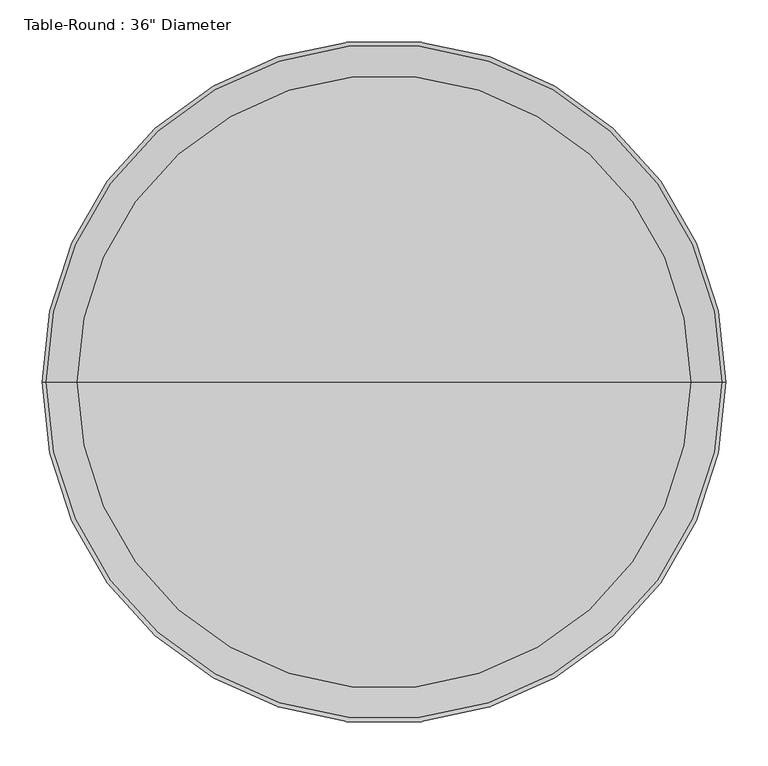
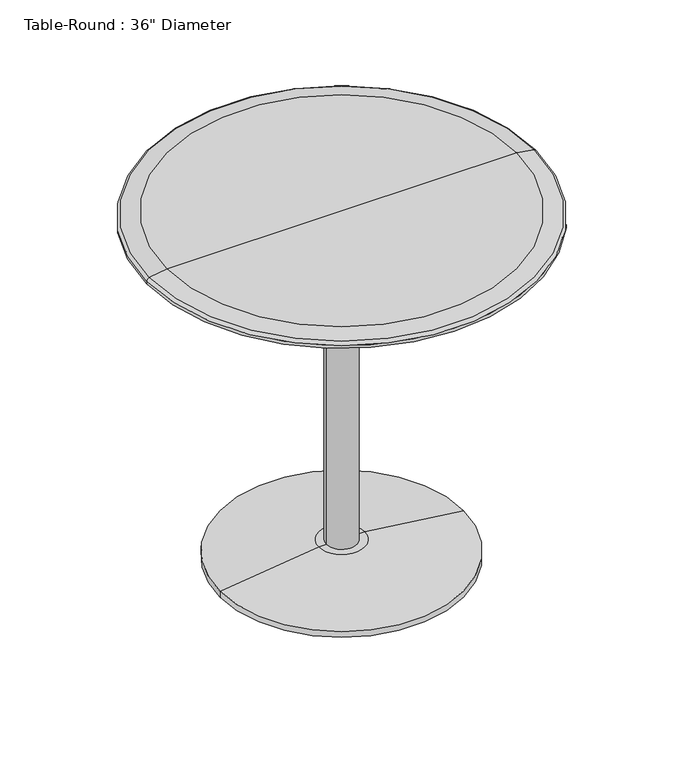
"""IFC4 building model written with IfcOpenShell, lengths in millimetres: furniture geometry."""

from ifc_helpers import new_model, si_unit, point, frame, origin, origin_2d, place, context, project, spatial, polyline, circle_curve, ellipse_curve, trimmed, segment, composite_curve, outline, extrude, source, transform, mapped, element, save
from ifc_brep_helpers import plane_surface, cylinder_surface, revolved_surface, advanced_brep


def furniture_eb3cba1b(model_context):
    return source(origin(), model_context, "Body", "SolidModel", [
        extrude(outline(composite_curve([segment(trimmed(circle_curve(origin_2d(), 31.75), [point((-31.75, 0.0))], [point((31.75, 0.0))], False, "CARTESIAN"), True, "CONTINUOUS"), segment(trimmed(circle_curve(origin_2d(), 31.75), [point((31.75, 0.0))], [point((-31.75, 0.0))], False, "CARTESIAN"), True, "CONTINUOUS")], self_intersect=False)), frame((0.0, 0.0, 38.1), z_axis=(0.0, 0.0, 1.0), x_axis=(1.0, 0.0, 0.0)), (0.0, 0.0, 1.0), 704.85),
        advanced_brep(
        [(0.0, 0.0, 742.95), (-406.4, 0.0, 742.95), (406.4, 0.0, 742.95), (364.5011364, 0.0, 762.0), (-364.5011364, 0.0, 762.0), (0.0, 0.0, 762.0), (401.1526659, 0.0, 755.5373465), (-401.1526659, 0.0, 755.5373465), (406.4, 0.0, 749.2838172), (-406.4, 0.0, 749.2838172)],
        [
            (0, 1),
            (1, 2, circle_curve(frame((0.0, 0.0, 742.95), z_axis=(0.0, 0.0, -1.0), x_axis=(-1.0, 0.0, 0.0)), 406.4)),
            (2, 0),
            (2, 1, circle_curve(frame((0.0, 0.0, 742.95), z_axis=(0.0, 0.0, -1.0), x_axis=(-1.0, 0.0, 0.0)), 406.4)),
            (3, 4, circle_curve(frame((0.0, 0.0, 762.0), z_axis=(0.0, 0.0, 1.0), x_axis=(-1.0, 0.0, 0.0)), 364.5011364)),
            (4, 5),
            (5, 3),
            (4, 3, circle_curve(frame((0.0, 0.0, 762.0), z_axis=(0.0, 0.0, 1.0), x_axis=(-1.0, 0.0, 0.0)), 364.5011364)),
            (6, 7, circle_curve(frame((0.0, 0.0, 755.5373465), z_axis=(0.0, 0.0, 1.0), x_axis=(-1.0, 0.0, 0.0)), 401.1526659)),
            (7, 4),
            (3, 6),
            (7, 6, circle_curve(frame((0.0, 0.0, 755.5373465), z_axis=(0.0, 0.0, 1.0), x_axis=(-1.0, 0.0, 0.0)), 401.1526659)),
            (8, 9, circle_curve(frame((0.0, 0.0, 749.2838172), z_axis=(0.0, 0.0, 1.0), x_axis=(-1.0, 0.0, 0.0)), 406.4)),
            (9, 7, circle_curve(frame((-400.05, 0.0, 749.2838172), z_axis=(0.0, 1.0, 0.0), x_axis=(1.0, 0.0, 0.0)), 6.35)),
            (6, 8, circle_curve(frame((400.05, 0.0, 749.2838172), z_axis=(0.0, 1.0, 0.0), x_axis=(-1.0, 0.0, 0.0)), 6.35)),
            (9, 8, circle_curve(frame((0.0, 0.0, 749.2838172), z_axis=(0.0, 0.0, 1.0), x_axis=(-1.0, 0.0, 0.0)), 406.4)),
            (1, 9),
            (8, 2),
        ],
        [
            plane_surface(frame((0.0, 0.0, 742.95), z_axis=(0.0, 0.0, -1.0), x_axis=(-1.0, 0.0, 0.0))),
            plane_surface(frame((0.0, 0.0, 762.0), z_axis=(0.0, 0.0, 1.0), x_axis=(-1.0, 0.0, 0.0))),
            revolved_surface(polyline([(-364.5011364, 0.0, 762.0), (-401.1526659, 0.0, 755.5373465)]), (0.0, 0.0, 838.2), (0.0, 0.0, -1.0)),
            revolved_surface(trimmed(ellipse_curve(frame((-400.05, 0.0, 749.2838172), z_axis=(0.0, -1.0, 0.0), x_axis=(1.0, 0.0, 0.0)), 6.35, 6.35), [point((-401.1526659, 0.0, 755.5373465))], [point((-406.4, 0.0, 749.2838172))], True, "CARTESIAN"), (0.0, 0.0, 838.2), (0.0, 0.0, -1.0)),
            cylinder_surface(frame((0.0, 0.0, 838.2), z_axis=(0.0, 0.0, -1.0), x_axis=(-1.0, 0.0, 0.0)), 406.4),
        ],
        [
            (0, [[1, 2, 3]]),
            (0, [[-3, 4, -1]]),
            (1, [[5, 6, 7]]),
            (1, [[8, -7, -6]]),
            (2, [[9, 10, -5, 11]]),
            (2, [[12, -11, -8, -10]]),
            (3, [[13, 14, -9, 15]]),
            (3, [[16, -15, -12, -14]]),
            (4, [[-2, 17, -13, 18]]),
            (4, [[-4, -18, -16, -17]]),
        ],
    ),
        advanced_brep(
        [(0.0, 0.0, 0.0), (-254.0, 0.0, 0.0), (254.0, 0.0, 0.0), (47.625, 0.0, 38.1), (-47.625, 0.0, 38.1), (0.0, 0.0, 38.1), (254.0, 0.0, 12.7), (-254.0, 0.0, 12.7)],
        [
            (0, 1),
            (1, 2, circle_curve(frame((0.0, 0.0, 0.0), z_axis=(0.0, 0.0, -1.0), x_axis=(-1.0, 0.0, 0.0)), 254.0)),
            (2, 0),
            (2, 1, circle_curve(frame((0.0, 0.0, 0.0), z_axis=(0.0, 0.0, -1.0), x_axis=(-1.0, 0.0, 0.0)), 254.0)),
            (3, 4, circle_curve(frame((0.0, 0.0, 38.1), z_axis=(0.0, 0.0, 1.0), x_axis=(-1.0, 0.0, 0.0)), 47.625)),
            (4, 5),
            (5, 3),
            (4, 3, circle_curve(frame((0.0, 0.0, 38.1), z_axis=(0.0, 0.0, 1.0), x_axis=(-1.0, 0.0, 0.0)), 47.625)),
            (6, 7, circle_curve(frame((0.0, 0.0, 12.7), z_axis=(0.0, 0.0, 1.0), x_axis=(-1.0, 0.0, 0.0)), 254.0)),
            (7, 4),
            (3, 6),
            (7, 6, circle_curve(frame((0.0, 0.0, 12.7), z_axis=(0.0, 0.0, 1.0), x_axis=(-1.0, 0.0, 0.0)), 254.0)),
            (1, 7),
            (6, 2),
        ],
        [
            plane_surface(frame((0.0, 0.0, 0.0), z_axis=(0.0, 0.0, -1.0), x_axis=(-1.0, 0.0, 0.0))),
            plane_surface(frame((0.0, 0.0, 38.1), z_axis=(0.0, 0.0, 1.0), x_axis=(-1.0, 0.0, 0.0))),
            revolved_surface(polyline([(-47.625, 0.0, 38.1), (-254.0, 0.0, 12.7)]), (0.0, 0.0, 215.9), (0.0, 0.0, -1.0)),
            cylinder_surface(frame((0.0, 0.0, 215.9), z_axis=(0.0, 0.0, -1.0), x_axis=(-1.0, 0.0, 0.0)), 254.0),
        ],
        [
            (0, [[1, 2, 3]]),
            (0, [[-3, 4, -1]]),
            (1, [[5, 6, 7]]),
            (1, [[8, -7, -6]]),
            (2, [[9, 10, -5, 11]]),
            (2, [[12, -11, -8, -10]]),
            (3, [[-2, 13, -9, 14]]),
            (3, [[-4, -14, -12, -13]]),
        ],
    ),
    ])


if __name__ == "__main__":
    model = new_model("IFC4")
    model_context = context("Model", 3, world=origin())
    ifc_project = project(units=[si_unit("LENGTHUNIT", "METRE", prefix="MILLI")], contexts=[model_context])
    site = spatial("IfcSite", under=ifc_project)
    building = spatial("IfcBuilding", under=site)
    placement = place(None, origin())
    furniture_shape = furniture_eb3cba1b(model_context)
    element("IfcFurniture", 1, ObjectType="Table-Round : 36\" Diameter", at=placement, inside=building, context=model_context, shape_type="MappedRepresentation", body=[
        mapped(furniture_shape, transform((0.0, 0.0, 0.0), x_axis=(1.0, 0.0, 0.0), y_axis=(0.0, 1.0, 0.0), z_axis=(0.0, 0.0, 1.0))),
    ])
    save(model, "model.ifc")

# Revit data of these elements
# Type "Table-Round : 36\" Diameter"
#   Assembly Code = "E2020200"
#   Base Radius = 0' - 10"
#   Height = 2' - 6"
#   Radius = 1' - 4"
#   Base Material = Steel, Chrome Plated
#   Top Material = Birch
#   Default Elevation = 0
# Element 1 (IfcFurniture, "Table-Round : 36\" Diameter")
#   Materials on its faces: "Steel, Chrome Plated", "Birch"
# Materials
#   "Steel, Chrome Plated": class "Metal", colour RGB 17 17 17, transparency 0, Description = "Chromiuim plated steel", Cost = 0
#   "Birch": class "Wood", colour RGB 224 178 126, transparency 0, Description = "Betula Alleghaniensis", Cost = 0
